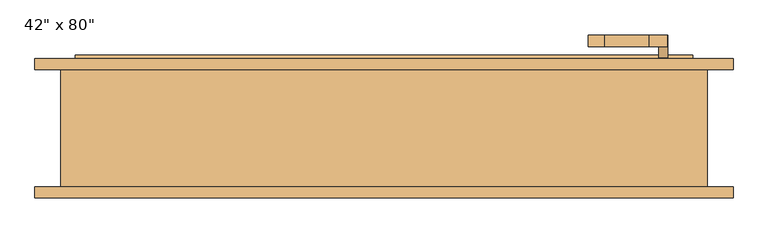
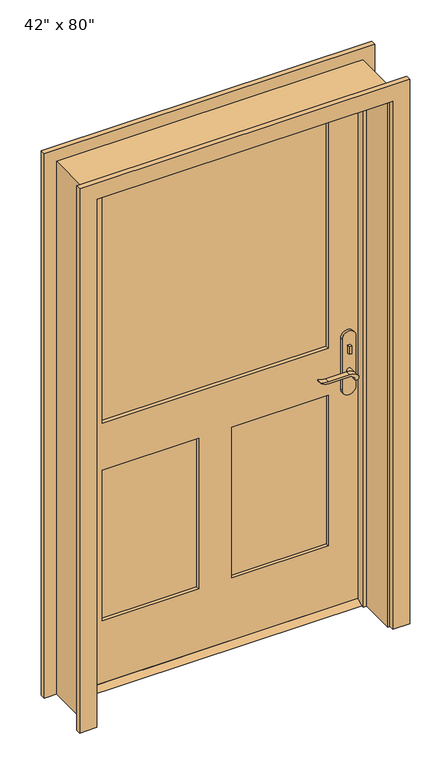
"""IFC4 building model written with IfcOpenShell, lengths in millimetres: door geometry."""

from ifc_helpers import new_model, si_unit, point, frame, frame_2d, origin, place, context, project, spatial, polyline, circle_curve, trimmed, segment, composite_curve, outline, extrude, faceted_brep, source, transform, mapped, element, save


def door_e0076512(model_context):
    return source(origin(), model_context, "Body", "SolidModel", [
        extrude(outline(polyline([(63.5, 12.7), (98.425, 12.7), (123.825, 0.0), (38.1, 0.0), (63.5, 12.7)])), frame((-533.4, 0.0, 0.0), z_axis=(1.0, 0.0, 0.0), x_axis=(0.0, 1.0, 0.0)), (0.0, 0.0, 1.0), 1066.8),
        extrude(outline(polyline([(487.6, 43.5), (477.6, 43.5), (477.6, 53.5), (487.6, 53.5), (487.6, 43.5)])), frame((0.0, 0.0, 981.9), z_axis=(0.0, 0.0, 1.0), x_axis=(1.0, 0.0, 0.0)), (0.0, 0.0, 1.0), 30.0),
        extrude(outline(composite_curve([segment(trimmed(circle_curve(frame_2d((996.9, 482.6)), 8.0), [point((996.9, 474.6))], [point((996.9, 490.6))], False, "CARTESIAN"), True, "CONTINUOUS"), segment(trimmed(circle_curve(frame_2d((996.9, 482.6)), 8.0), [point((996.9, 490.6))], [point((996.9, 474.6))], False, "CARTESIAN"), True, "CONTINUOUS")], self_intersect=False)), frame((0.0, 108.425, 0.0), z_axis=(0.0, 1.0, 0.0), x_axis=(0.0, 0.0, 1.0)), (0.0, 0.0, 1.0), 10.0),
        extrude(outline(composite_curve([segment(trimmed(circle_curve(frame_2d((897.1555521, 458.9324871)), 37.2832219), [point((919.0523287, 489.1081363))], [point((934.4, 457.2325667))], False, "CARTESIAN"), True, "CONTINUOUS"), segment(polyline([(934.4, 457.2325667), (934.4, 380.9564091)]), True, "CONTINUOUS"), segment(trimmed(circle_curve(frame_2d((1017.6850638, 381.0227909)), 83.2850902), [point((934.4, 380.9564091))], [point((939.4, 352.6))], True, "CARTESIAN"), True, "CONTINUOUS"), segment(polyline([(939.4, 352.6), (936.6135558, 352.6)]), True, "CONTINUOUS"), segment(trimmed(circle_curve(frame_2d((986.6709207, 384.5396612)), 59.3791355), [point((936.6135558, 352.6))], [point((927.4, 380.9564091))], False, "CARTESIAN"), True, "CONTINUOUS"), segment(polyline([(927.4, 380.9564091), (927.4, 457.2138099)]), True, "CONTINUOUS"), segment(trimmed(circle_curve(frame_2d((909.2738613, 457.2138099)), 18.1261387), [point((927.4, 457.2138099))], [point((914.4, 474.6))], True, "CARTESIAN"), True, "CONTINUOUS"), segment(trimmed(circle_curve(frame_2d((914.4, 482.6)), 8.0), [point((914.4, 474.6))], [point((919.0523287, 489.1081363))], False, "CARTESIAN"), True, "CONTINUOUS")], self_intersect=False)), frame((0.0, 3.5, 0.0), z_axis=(0.0, 1.0, 0.0), x_axis=(0.0, 0.0, 1.0)), (0.0, 0.0, 1.0), 20.0),
        extrude(outline(composite_curve([segment(trimmed(circle_curve(frame_2d((914.4, 482.6)), 8.0), [point((914.3999903, 474.6))], [point((919.0523287, 489.1081363))], False, "CARTESIAN"), True, "CONTINUOUS"), segment(trimmed(circle_curve(frame_2d((897.1555521, 458.9324871)), 37.2832219), [point((919.0523287, 489.1081363))], [point((934.4, 457.2325667))], False, "CARTESIAN"), True, "CONTINUOUS"), segment(polyline([(934.4, 457.2325667), (934.4, 380.9564091)]), True, "CONTINUOUS"), segment(trimmed(circle_curve(frame_2d((1017.6850638, 381.0227909)), 83.2850902), [point((934.4, 380.9564091))], [point((939.4, 352.6))], True, "CARTESIAN"), True, "CONTINUOUS"), segment(polyline([(939.4, 352.6), (936.6135558, 352.6)]), True, "CONTINUOUS"), segment(trimmed(circle_curve(frame_2d((986.6709207, 384.5396612)), 59.3791355), [point((936.6135558, 352.6))], [point((927.4, 380.9564091))], False, "CARTESIAN"), True, "CONTINUOUS"), segment(polyline([(927.4, 380.9564091), (927.4, 457.2138122)]), True, "CONTINUOUS"), segment(trimmed(circle_curve(frame_2d((909.2738682, 457.2138122)), 18.1261318), [point((927.4, 457.2138122))], [point((914.3999903, 474.6))], True, "CARTESIAN"), True, "CONTINUOUS")], self_intersect=False)), frame((0.0, 138.425, 0.0), z_axis=(0.0, 1.0, 0.0), x_axis=(0.0, 0.0, 1.0)), (0.0, 0.0, 1.0), 20.0),
        extrude(outline(composite_curve([segment(trimmed(circle_curve(frame_2d((914.4, 482.6)), 8.0), [point((914.4, 474.6))], [point((914.4, 490.6))], False, "CARTESIAN"), True, "CONTINUOUS"), segment(trimmed(circle_curve(frame_2d((914.4, 482.6)), 8.0), [point((914.4, 490.6))], [point((914.4, 474.6))], False, "CARTESIAN"), True, "CONTINUOUS")], self_intersect=False)), frame((0.0, 23.5, 0.0), z_axis=(0.0, 1.0, 0.0), x_axis=(0.0, 0.0, 1.0)), (0.0, 0.0, 1.0), 30.0),
        extrude(outline(composite_curve([segment(trimmed(circle_curve(frame_2d((914.4, 482.6)), 8.0), [point((914.4, 474.6))], [point((914.4, 490.6))], False, "CARTESIAN"), True, "CONTINUOUS"), segment(trimmed(circle_curve(frame_2d((914.4, 482.6)), 8.0), [point((914.4, 490.6))], [point((914.4, 474.6))], False, "CARTESIAN"), True, "CONTINUOUS")], self_intersect=False)), frame((0.0, 108.425, 0.0), z_axis=(0.0, 1.0, 0.0), x_axis=(0.0, 0.0, 1.0)), (0.0, 0.0, 1.0), 30.0),
        extrude(outline(composite_curve([segment(polyline([(844.4, 507.6), (1039.4, 507.6)]), True, "CONTINUOUS"), segment(trimmed(circle_curve(frame_2d((1039.4, 482.6)), 25.0), [point((1039.4, 507.6))], [point((1039.4, 457.6))], False, "CARTESIAN"), True, "CONTINUOUS"), segment(polyline([(1039.4, 457.6), (844.4, 457.6)]), True, "CONTINUOUS"), segment(trimmed(circle_curve(frame_2d((844.4, 482.6)), 25.0), [point((844.4, 457.6))], [point((844.4, 507.6))], False, "CARTESIAN"), True, "CONTINUOUS")], self_intersect=False)), frame((0.0, 53.5, 0.0), z_axis=(0.0, 1.0, 0.0), x_axis=(0.0, 0.0, 1.0)), (0.0, 0.0, 1.0), 10.0),
        extrude(outline(composite_curve([segment(polyline([(844.4, 507.6), (1039.4, 507.6)]), True, "CONTINUOUS"), segment(trimmed(circle_curve(frame_2d((1039.4, 482.6)), 25.0), [point((1039.4, 507.6))], [point((1039.4, 457.6))], False, "CARTESIAN"), True, "CONTINUOUS"), segment(polyline([(1039.4, 457.6), (844.4, 457.6)]), True, "CONTINUOUS"), segment(trimmed(circle_curve(frame_2d((844.4, 482.6)), 25.0), [point((844.4, 457.6))], [point((844.4, 507.6))], False, "CARTESIAN"), True, "CONTINUOUS")], self_intersect=False)), frame((0.0, 98.425, 0.0), z_axis=(0.0, 1.0, 0.0), x_axis=(0.0, 0.0, 1.0)), (0.0, 0.0, 1.0), 10.0),
        extrude(outline(polyline([(2032.0, -533.4), (12.7, -533.4), (12.7, 533.4), (2032.0, 533.4), (2032.0, -533.4)]), holes=[polyline([(1016.0, -412.75), (1911.35, -412.75), (1911.35, 412.75), (1016.0, 412.75), (1016.0, -412.75)]), polyline([(835.025, -60.325), (254.0, -60.325), (254.0, -412.75), (835.025, -412.75), (835.025, -60.325)]), polyline([(835.025, 412.75), (254.0, 412.75), (254.0, 60.325), (835.025, 60.325), (835.025, 412.75)])]), frame((0.0, 63.5, 0.0), z_axis=(0.0, 1.0, 0.0), x_axis=(0.0, 0.0, 1.0)), (0.0, 0.0, 1.0), 34.925),
        faceted_brep([(558.8, 98.425, 0.0), (558.8, -104.775, 0.0), (533.4, -104.775, 0.0), (533.4, 28.575, 0.0), (520.7, 28.575, 0.0), (520.7, 63.5, 0.0), (533.4, 63.5, 0.0), (533.4, 98.425, 0.0), (558.8, 98.425, 2057.4), (558.8, -104.775, 2057.4), (-558.8, -104.775, 2057.4), (-558.8, -104.775, 0.0), (-533.4, -104.775, 0.0), (-533.4, -104.775, 2032.0), (533.4, -104.775, 2032.0), (533.4, 28.575, 2032.0), (-533.4, 28.575, 2032.0), (-533.4, 28.575, 0.0), (-520.7, 28.575, 0.0), (-520.7, 28.575, 2019.3), (520.7, 28.575, 2019.3), (520.7, 63.5, 2019.3), (-520.7, 63.5, 2019.3), (-520.7, 63.5, 0.0), (-533.4, 63.5, 0.0), (-533.4, 63.5, 2032.0), (533.4, 63.5, 2032.0), (533.4, 98.425, 2032.0), (-533.4, 98.425, 2032.0), (-533.4, 98.425, 0.0), (-558.8, 98.425, 0.0), (-558.8, 98.425, 2057.4)], [[[0, 1, 2, 3, 4, 5, 6, 7]], [[1, 0, 8, 9]], [[2, 1, 9, 10, 11, 12, 13, 14]], [[3, 2, 14, 15]], [[4, 3, 15, 16, 17, 18, 19, 20]], [[5, 4, 20, 21]], [[6, 5, 21, 22, 23, 24, 25, 26]], [[7, 6, 26, 27]], [[0, 7, 27, 28, 29, 30, 31, 8]], [[9, 8, 31, 10]], [[15, 14, 13, 16]], [[21, 20, 19, 22]], [[27, 26, 25, 28]], [[30, 29, 24, 23, 18, 17, 12, 11]], [[10, 31, 30, 11]], [[16, 13, 12, 17]], [[22, 19, 18, 23]], [[28, 25, 24, 29]]]),
        extrude(outline(polyline([(-60.325, 75.1416667), (-412.75, 75.1416667), (-412.75, 86.7833333), (-60.325, 86.7833333), (-60.325, 75.1416667)])), frame((0.0, 0.0, 254.0), z_axis=(0.0, 0.0, 1.0), x_axis=(1.0, 0.0, 0.0)), (0.0, 0.0, 1.0), 581.025),
        extrude(outline(polyline([(412.75, 75.1416667), (60.325, 75.1416667), (60.325, 86.7833333), (412.75, 86.7833333), (412.75, 75.1416667)])), frame((0.0, 0.0, 254.0), z_axis=(0.0, 0.0, 1.0), x_axis=(1.0, 0.0, 0.0)), (0.0, 0.0, 1.0), 581.025),
        extrude(outline(polyline([(412.75, 77.47), (-412.75, 77.47), (-412.75, 84.455), (412.75, 84.455), (412.75, 77.47)])), frame((0.0, 0.0, 1016.0), z_axis=(0.0, 0.0, 1.0), x_axis=(1.0, 0.0, 0.0)), (0.0, 0.0, 1.0), 895.35),
        extrude(outline(polyline([(0.0, -603.25), (0.0, -539.75), (2038.35, -539.75), (2038.35, 539.75), (0.0, 539.75), (0.0, 603.25), (2101.85, 603.25), (2101.85, -603.25), (0.0, -603.25)])), frame((0.0, -123.825, 0.0), z_axis=(0.0, 1.0, 0.0), x_axis=(0.0, 0.0, 1.0)), (0.0, 0.0, 1.0), 19.05),
        extrude(outline(polyline([(0.0, -603.25), (0.0, -539.75), (2038.35, -539.75), (2038.35, 539.75), (0.0, 539.75), (0.0, 603.25), (2101.85, 603.25), (2101.85, -603.25), (0.0, -603.25)])), frame((0.0, 98.425, 0.0), z_axis=(0.0, 1.0, 0.0), x_axis=(0.0, 0.0, 1.0)), (0.0, 0.0, 1.0), 19.05),
    ])


if __name__ == "__main__":
    model = new_model("IFC4")
    model_context = context("Model", 3, world=origin())
    ifc_project = project(units=[si_unit("LENGTHUNIT", "METRE", prefix="MILLI")], contexts=[model_context])
    site = spatial("IfcSite", under=ifc_project)
    building = spatial("IfcBuilding", under=site)
    placement = place(None, origin())
    door_shape = door_e0076512(model_context)
    element("IfcDoor", 1, ObjectType="42\" x 80\"", at=placement, inside=building, context=model_context, shape_type="MappedRepresentation", body=[
        mapped(door_shape, transform((0.0, 0.0, 0.0), x_axis=(1.0, 0.0, 0.0), y_axis=(0.0, 1.0, 0.0), z_axis=(0.0, 0.0, 1.0))),
    ])
    save(model, "model.ifc")

# Revit data of these elements
# Type "42\" x 80\""
#   Type Mark = "9"
#   Assembly Code = "B2030100"
#   Analytic Construction = "French door, wood frame with single glass"
#   Top Rail = 0' - 4 3/4"
#   Threshold Offset [instance default] = 0' - 0 1/2"
#   Thickness = 0' - 1 3/8"
#   Thermal Resistance (R) = 1.0696 (h·ft²·°F)/BTU
#   Swing Angle [instance default] = 90.00°
#   Stiles = 0' - 4 3/4"
#   Rough Width = 3' - 8"
#   Rough Height = 6' - 9"
#   Lock Rail = 0' - 7 1/8"
#   Height = 6' - 8"
#   Width = 3' - 6"
#   Heat Transfer Coefficient (U) = 0.9350 BTU/(h·ft²·°F)
#   Door Offset [instance default] = 0' - 0"
#   Bottom Rail = 0' - 9 1/2"
#   Threshold [instance default] = yes
#   Function = 1
#   Exterior Trim [instance default] = yes
#   Trim Material = Cherry
#   Threshold Material = Cherry
#   Panel Material = Cherry
#   Glazing = Glass
#   Frame Material = Cherry
#   Door Handle Material = Aluminum
#   Visual Light Transmittance = 0
#   Solar Heat Gain Coefficient = 0
#   Wall Closure = (empty or 0)
#   Construction Type = (empty or 0)
# Element 1 (IfcDoor, "42\" x 80\"")
#   Materials on its faces: "Cherry", "Aluminum", "Glass"
# Materials
#   "Cherry": class "Wood", colour RGB 226 177 128, transparency 0, Description = "Prunus Serotina", Cost = 0
#   "Glass": class "Glass", colour RGB 0 128 192, transparency 0.75, Description = "Soda Lime Glass", Cost = 0
#   "Aluminum": class "Metal", colour RGB 247 247 247, transparency 0, Description = "Aluminum 6061", Cost = 0
